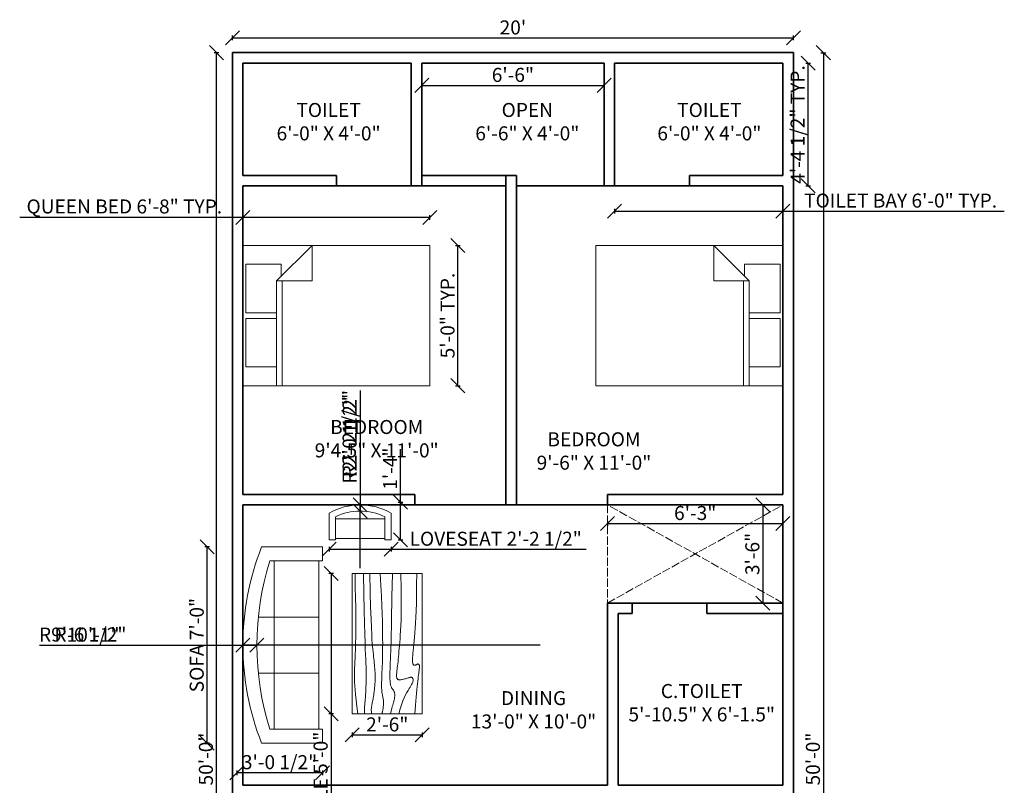
# Model space of a CAD drawing. Units: inches. Extents: x 2598 to 3019, y 330 to 985.
# Tile 2 of 2: x 2598 to 3019, y 657 to 985. Entities that reach past the tile are written whole.
import ezdxf

# ---------------------------------------------------------------- set-up
doc = ezdxf.new("R2010")
doc.units = ezdxf.units.IN
doc.linetypes.add('ACAD_ISO02W100', pattern=[15, 12, -3])
for name, color, linetype, lineweight in [('A-ANNO-DIMS', 2, 'Continuous', 13), ('A-AREA-IDEN', 114, 'Continuous', 18), ('A-FLOR-OVHD', 8, 'ACAD_ISO02W100', 13), ('A-FURN', 8, 'Continuous', 18), ('A-WALL', 7, 'Continuous', 35)]:
    doc.layers.add(name, color=color, linetype=linetype, lineweight=lineweight)
doc.styles.get("Standard").update_dxf_attribs({"font": 'arial.ttf'})
doc.dimstyles.new('ISO-25', dxfattribs={"dimtxt": 6, "dimasz": 6, "dimexe": 1, "dimexo": 3, "dimtad": 1, "dimlunit": 3, "dimtxsty": 'Standard', "dimblk": 'OBLIQUE', "dimcen": 2.5, "dimclrt": 6, "dimadec": 0, "dimazin": 0, "dimtfac": 1, "dimtmove": 0, "dimatfit": 3, "dimfxl": 1, "dimfxlon": 1, "dimarcsym": 0})

# ---------------------------------------------------------------- blocks, each defined once
blk = doc.blocks.new('_Oblique')
at = {"color": 0, "linetype": 'ByBlock', "lineweight": -2}
blk.add_line((-0.5, -0.5), (0.5, 0.5), dxfattribs=at)
blk = doc.blocks.new('*D2')
at = {"layer": 'A-ANNO-DIMS', "color": 0, "lineweight": -2, "transparency": 16777216}
for p, q in [((2770.06, 957.96), (2770.06, 955.96)), ((2770.06, 956.96), (2848.06, 956.96)), ((2848.06, 957.96), (2848.06, 955.96))]:
    blk.add_line(p, q, dxfattribs=at)
at = {"layer": 'Defpoints', "color": 0, "transparency": 16777216}
for p in [(2770.06, 966.44), (2848.06, 966.44), (2848.06, 956.96)]:
    blk.add_point(p, dxfattribs=at)
at = {"layer": 'A-ANNO-DIMS', "color": 0, "lineweight": -2, "transparency": 16777216, "xscale": 6, "yscale": 6, "zscale": 6, "rotation": 180}
blk.add_blockref('_Oblique', (2770.06, 956.96), dxfattribs=at)
at = {"layer": 'A-ANNO-DIMS', "color": 0, "lineweight": -2, "transparency": 16777216, "xscale": 6, "yscale": 6, "zscale": 6}
blk.add_blockref('_Oblique', (2848.06, 956.96), dxfattribs=at)
at = {"layer": 'A-ANNO-DIMS', "color": 0, "transparency": 16777216, "insert": (2809.06, 960.65), "char_height": 6, "attachment_point": 5}
blk.add_mtext('6\'-6"', dxfattribs=at)
blk = doc.blocks.new('*D3')
at = {"layer": 'A-ANNO-DIMS', "color": 0, "lineweight": -2, "transparency": 16777216}
for p, q in [((2689.06, 976.27), (2689.06, 978.27)), ((2929.06, 976.27), (2929.06, 978.27)), ((2689.06, 977.27), (2929.06, 977.27))]:
    blk.add_line(p, q, dxfattribs=at)
at = {"layer": 'Defpoints', "color": 0, "transparency": 16777216}
for p in [(2929.06, 977.27), (2689.06, 970.94), (2929.06, 970.94)]:
    blk.add_point(p, dxfattribs=at)
at = {"layer": 'A-ANNO-DIMS', "color": 0, "lineweight": -2, "transparency": 16777216, "xscale": 6, "yscale": 6, "zscale": 6, "rotation": 180}
blk.add_blockref('_Oblique', (2689.06, 977.27), dxfattribs=at)
at = {"layer": 'A-ANNO-DIMS', "color": 0, "lineweight": -2, "transparency": 16777216, "xscale": 6, "yscale": 6, "zscale": 6}
blk.add_blockref('_Oblique', (2929.06, 977.27), dxfattribs=at)
at = {"layer": 'A-ANNO-DIMS', "color": 0, "transparency": 16777216, "insert": (2809.06, 980.96), "char_height": 6, "attachment_point": 5}
blk.add_mtext("20'", dxfattribs=at)
blk = doc.blocks.new('*D4')
at = {"layer": 'A-ANNO-DIMS', "color": 0, "lineweight": -2, "transparency": 16777216}
for p, q in [((2940.88, 970.94), (2942.88, 970.94)), ((2941.88, 970.94), (2941.88, 366.44)), ((2940.88, 366.44), (2942.88, 366.44))]:
    blk.add_line(p, q, dxfattribs=at)
at = {"layer": 'Defpoints', "color": 0, "transparency": 16777216}
for p in [(2929.06, 970.94), (2929.06, 366.44), (2941.88, 366.44)]:
    blk.add_point(p, dxfattribs=at)
at = {"layer": 'A-ANNO-DIMS', "color": 0, "lineweight": -2, "transparency": 16777216, "xscale": 6, "yscale": 6, "zscale": 6}
for p, rotation in [((2941.88, 970.94), 90), ((2941.88, 366.44), 270)]:
    blk.add_blockref('_Oblique', p, dxfattribs=dict(at, rotation=rotation))
at = {"layer": 'A-ANNO-DIMS', "color": 0, "transparency": 16777216, "insert": (2938.2, 668.69), "char_height": 6, "attachment_point": 5, "rotation": 90}
blk.add_mtext('50\'-0"', dxfattribs=at)
blk = doc.blocks.new('*D7')
at = {"layer": 'A-ANNO-DIMS', "color": 0, "lineweight": -2, "transparency": 16777216}
for p, q in [((2849.56, 770.49), (2849.56, 768.49)), ((2849.56, 769.49), (2924.56, 769.49)), ((2924.56, 770.49), (2924.56, 768.49))]:
    blk.add_line(p, q, dxfattribs=at)
at = {"layer": 'Defpoints', "color": 0, "transparency": 16777216}
for p in [(2849.56, 777.44), (2924.56, 777.44), (2924.56, 769.49)]:
    blk.add_point(p, dxfattribs=at)
at = {"layer": 'A-ANNO-DIMS', "color": 0, "lineweight": -2, "transparency": 16777216, "xscale": 6, "yscale": 6, "zscale": 6, "rotation": 180}
blk.add_blockref('_Oblique', (2849.56, 769.49), dxfattribs=at)
at = {"layer": 'A-ANNO-DIMS', "color": 0, "lineweight": -2, "transparency": 16777216, "xscale": 6, "yscale": 6, "zscale": 6}
blk.add_blockref('_Oblique', (2924.56, 769.49), dxfattribs=at)
at = {"layer": 'A-ANNO-DIMS', "color": 0, "transparency": 16777216, "insert": (2887.06, 773.18), "char_height": 6, "attachment_point": 5}
blk.add_mtext('6\'-3"', dxfattribs=at)
blk = doc.blocks.new('*D8')
at = {"layer": 'A-ANNO-DIMS', "color": 0, "lineweight": -2, "transparency": 16777216}
for p, q in [((2916.98, 777.44), (2914.98, 777.44)), ((2915.98, 777.44), (2915.98, 735.44)), ((2916.98, 735.44), (2914.98, 735.44))]:
    blk.add_line(p, q, dxfattribs=at)
at = {"layer": 'Defpoints', "color": 0, "transparency": 16777216}
for p in [(2924.56, 777.44), (2915.98, 735.44), (2924.56, 735.44)]:
    blk.add_point(p, dxfattribs=at)
at = {"layer": 'A-ANNO-DIMS', "color": 0, "lineweight": -2, "transparency": 16777216, "xscale": 6, "yscale": 6, "zscale": 6}
for p, rotation in [((2915.98, 777.44), 90), ((2915.98, 735.44), 270)]:
    blk.add_blockref('_Oblique', p, dxfattribs=dict(at, rotation=rotation))
at = {"layer": 'A-ANNO-DIMS', "color": 0, "transparency": 16777216, "insert": (2912.29, 756.44), "char_height": 6, "attachment_point": 5, "rotation": 90}
blk.add_mtext('3\'-6"', dxfattribs=at)
blk = doc.blocks.new('Bed - Queen')
for p, q in [((0, -80.00003), (0, 0)), ((0, 0), (59.99999, 0)), ((59.99999, 0), (59.99999, -80.00003)), ((7.99999, -1.2), (28.79998, -1.2)), ((7.99999, -14.4), (7.99999, -1.2)), ((28.79998, -1.2), (28.79998, -14.4)), ((31.19999, -1.2), (51.99999, -1.2)), ((31.19999, -14.4), (31.19999, -1.2)), ((51.99999, -1.2), (51.99999, -16.4)), ((0, -14.4), (44.8, -14.4)), ((44.8, -16.8), (0, -16.8)), ((59.99999, -29.6), (44.8, -14.4)), ((44.8, -14.4), (44.8, -29.6)), ((51.99999, -16.4), (46.79936, -16.4)), ((44.8, -29.6), (59.99999, -29.6)), ((59.99999, -80.00003), (0, -80.00003))]:
    blk.add_line(p, q)
blk = doc.blocks.new('Sofa - Roundback 7 ft.')
for p, q in [((-12.00002, -32.4421), (-12.00003, -6.5971)), ((11.99997, -32.4421), (11.99998, -6.5971)), ((-36.000027, -34), (-36.000027, -11.4696)), ((35.99998, -34), (35.99998, -11.4696)), ((-35.999844, -13.3819), (35.9998, -13.3819)), ((-36.000027, -32.4421), (35.99998, -32.4421))]:
    blk.add_line(p, q)
for points in [[(-36.000027, -34), (-42.000027, -34), (-42.000027, -8)], [(41.99998, -8), (41.99998, -34), (35.99998, -34)]]:
    blk.add_lwpolyline(points)
for centre, radius, start, end in [((0, -114.25), 114.25, 68.43141, 111.5686), ((-0.00001, -127.1968), 121.1968, 72.72033, 107.2797)]:
    blk.add_arc(centre, radius, start, end)
blk = doc.blocks.new('Sofa - Roundback Loveseat 5 ft.')
for p, q in [((0, -32.44198), (0, -5.99998)), ((-24, -33.99998), (-24, -11.46958)), ((-23.9998, -13.38178), (23.99986, -13.38178)), ((24.00004, -33.99998), (24.00004, -11.46958)), ((-24, -32.44198), (24.00004, -32.44198))]:
    blk.add_line(p, q)
for points in [[(-24, -33.99998), (-30, -33.99998), (-30, -7.99998)], [(30.00004, -7.99998), (30.00004, -33.99998), (24.00004, -33.99998)]]:
    blk.add_lwpolyline(points)
for centre, radius, start, end in [((0, -60.24998), 60.24998, 60.13715, 119.8628), ((0, -61.38438), 55.38444, 64.32083, 115.6792)]:
    blk.add_arc(centre, radius, start, end)
blk = doc.blocks.new('Table - Rectangular Woodgrain 60 x 30 in.')
for p, q in [((0, 0), (0, -30)), ((60, 0), (0, 0)), ((60, -30), (60, 0)), ((0, -30), (60, -30))]:
    blk.add_line(p, q)
for points in [[(0, -2.4), (4.8155, -2.418), (9.0302, -2.4688), (12.709, -2.5477), (15.9167, -2.65), (18.7181, -2.7711), (21.1781, -2.9063), (23.3616, -3.0508), (25.3333, -3.2), (27.1477, -3.3495), (28.8172, -3.4958), (30.3437, -3.636), (31.7291, -3.7667), (32.9756, -3.8849), (34.0849, -3.9875), (35.059, -4.0714), (35.9, -4.1334), (36.6114, -4.1711), (37.2041, -4.1854), (37.6906, -4.1779), (38.0833, -4.15), (38.3948, -4.1034), (38.6375, -4.0396), (38.8239, -3.9602), (38.9666, -3.8667), (39.0764, -3.7608), (39.1573, -3.6448), (39.2116, -3.521), (39.2416, -3.3917), (39.2498, -3.2593), (39.2385, -3.1261), (39.21, -2.9944), (39.1666, -2.8667), (39.111, -2.7447), (39.0468, -2.6281), (38.978, -2.5163), (38.9083, -2.4083), (38.8418, -2.3035), (38.7823, -2.201), (38.7337, -2.1001), (38.7, -2), (38.6844, -1.9003), (38.6875, -1.8021), (38.7094, -1.707), (38.75, -1.6167), (38.8094, -1.5326), (38.8875, -1.4563), (38.9844, -1.3893), (39.1, -1.3333), (39.2351, -1.2896), (39.3937, -1.2583), (39.5804, -1.2396), (39.8, -1.2333), (40.057, -1.2396), (40.3562, -1.2583), (40.7023, -1.2896), (41.1, -1.3333), (41.5547, -1.3895), (42.0755, -1.4573), (42.6721, -1.5361), (43.3542, -1.625), (44.1316, -1.7233), (45.014, -1.8302), (46.0114, -1.9449), (47.1333, -2.0667), (48.3862, -2.1947), (49.7625, -2.3281), (51.2513, -2.4663), (52.8416, -2.6083), (54.5226, -2.7535), (56.2833, -2.9011), (58.1127, -3.0501), (60, -3.2)], [(0, -9.2), (6.5759, -9.0858), (11.9385, -9.0365), (16.2527, -9.0418), (19.6833, -9.0917), (22.3952, -9.1759), (24.5531, -9.2844), (26.322, -9.4069), (27.8666, -9.5333), (29.3241, -9.6553), (30.7203, -9.7719), (32.0532, -9.8837), (33.3208, -9.9917), (34.5213, -10.0965), (35.6526, -10.199), (36.7128, -10.2999), (37.7, -10.4), (38.6129, -10.4996), (39.4531, -10.5969), (40.223, -10.6895), (40.925, -10.775), (41.5613, -10.8512), (42.1344, -10.9156), (42.6465, -10.966), (43.1, -11), (43.4976, -11.0158), (43.8437, -11.0136), (44.143, -10.9942), (44.4, -10.9583), (44.6195, -10.9069), (44.8062, -10.8406), (44.9648, -10.7603), (45.1, -10.6667), (45.2155, -10.5598), (45.3114, -10.4365), (45.3871, -10.2929), (45.4416, -10.125), (45.4743, -9.929), (45.4844, -9.7011), (45.4709, -9.4371), (45.4333, -9.1333), (45.3716, -8.7883), (45.2896, -8.4104), (45.1919, -8.0107), (45.0833, -7.6), (44.9685, -7.1893), (44.8521, -6.7896), (44.7388, -6.4117), (44.6333, -6.0667), (44.54, -5.7628), (44.4614, -5.4979), (44.4001, -5.2675), (44.3583, -5.0667), (44.3384, -4.8909), (44.3427, -4.7354), (44.3736, -4.5956), (44.4333, -4.4667), (44.5236, -4.3453), (44.6427, -4.2333), (44.7884, -4.1339), (44.9583, -4.05), (45.1501, -3.9849), (45.3614, -3.9417), (45.59, -3.9234), (45.8333, -3.9333), (46.0915, -3.9749), (46.3734, -4.0531), (46.6906, -4.1736), (47.0542, -4.3417), (47.4756, -4.5629), (47.9661, -4.8427), (48.5372, -5.1866), (49.2, -5.6), (49.9676, -6.0844), (50.8594, -6.625), (51.8965, -7.2031), (53.1, -7.8), (54.491, -8.3969), (56.0906, -8.975), (57.9199, -9.5156), (60, -10)], [(0, -12.8), (5.1847, -12.9322), (9.6213, -13.0323), (13.3963, -13.1059), (16.5958, -13.1583), (19.3063, -13.1952), (21.614, -13.2219), (23.6054, -13.2439), (25.3666, -13.2667), (26.9728, -13.2947), (28.4531, -13.3281), (29.8256, -13.3663), (31.1083, -13.4083), (32.3191, -13.4535), (33.476, -13.501), (34.597, -13.5501), (35.7, -13.6), (36.7984, -13.6497), (37.8875, -13.6979), (38.9578, -13.743), (40, -13.7833), (41.0047, -13.8174), (41.9625, -13.8438), (42.864, -13.8607), (43.7, -13.8667), (44.4631, -13.8604), (45.1552, -13.8417), (45.7801, -13.8104), (46.3416, -13.7667), (46.8439, -13.7104), (47.2906, -13.6417), (47.6858, -13.5604), (48.0333, -13.4667), (48.3375, -13.3608), (48.6042, -13.2448), (48.8396, -13.121), (49.05, -12.9917), (49.2417, -12.8593), (49.4208, -12.7261), (49.5937, -12.5944), (49.7667, -12.4667), (49.9452, -12.3451), (50.1323, -12.2313), (50.3303, -12.1268), (50.5416, -12.0333), (50.7686, -11.9524), (51.0135, -11.8854), (51.2788, -11.8341), (51.5666, -11.8), (51.8785, -11.7843), (52.2116, -11.7865), (52.562, -11.8059), (52.926, -11.8417), (53.2998, -11.8931), (53.6795, -11.9594), (54.0614, -12.0397), (54.4416, -12.1333), (54.8223, -12.2401), (55.2293, -12.3625), (55.6942, -12.5037), (56.2489, -12.6667), (56.9251, -12.8547), (57.7545, -13.0708), (58.7689, -13.3182), (60, -13.6)], [(0, -18), (5.124, -17.7273), (9.6609, -17.5057), (13.6705, -17.3303), (17.2125, -17.1958), (20.3467, -17.0973), (23.1328, -17.0297), (25.6307, -16.9878), (27.9, -16.9667), (29.9928, -16.9617), (31.9302, -16.9703), (33.7254, -16.9907), (35.3917, -17.0208), (36.9423, -17.0588), (38.3906, -17.1026), (39.7499, -17.1503), (41.0333, -17.2), (42.2519, -17.2496), (43.4073, -17.2969), (44.4986, -17.3395), (45.525, -17.375), (46.4858, -17.4012), (47.3802, -17.4156), (48.2074, -17.416), (48.9667, -17.4), (49.6583, -17.3662), (50.2872, -17.3167), (50.8595, -17.2547), (51.3812, -17.1833), (51.8584, -17.1057), (52.2971, -17.025), (52.7034, -16.9443), (53.0833, -16.8667), (53.443, -16.7951), (53.789, -16.7313), (54.128, -16.6768), (54.4666, -16.6334), (54.8115, -16.6024), (55.1693, -16.5854), (55.5465, -16.5841), (55.95, -16.6), (56.3828, -16.6337), (56.8346, -16.6823), (57.2915, -16.7418), (57.7396, -16.8084), (58.165, -16.878), (58.5539, -16.9469), (58.8924, -17.0111), (59.1666, -17.0667), (59.3679, -17.1107), (59.5078, -17.1438), (59.6032, -17.1675), (59.6708, -17.1833), (59.7275, -17.193), (59.7901, -17.1979), (59.8753, -17.1998), (60, -17.2)], [(0, -22.4), (8.0098, -22.2501), (14.4094, -22.1011), (19.4168, -21.9535), (23.25, -21.8083), (26.1269, -21.6663), (28.2656, -21.5281), (29.884, -21.3947), (31.2, -21.2667), (32.3967, -21.1448), (33.5172, -21.0292), (34.5697, -20.9198), (35.5625, -20.8167), (36.5037, -20.7198), (37.4015, -20.6292), (38.2642, -20.5448), (39.1, -20.4667), (39.9164, -20.3951), (40.7187, -20.3313), (41.5117, -20.2768), (42.3, -20.2333), (43.0883, -20.2024), (43.8812, -20.1854), (44.6836, -20.1841), (45.5, -20.2), (46.3328, -20.234), (47.1747, -20.2844), (48.0163, -20.3488), (48.8479, -20.425), (49.66, -20.5106), (50.4429, -20.6031), (51.1872, -20.7004), (51.8833, -20.8), (52.5246, -20.8999), (53.1166, -20.9995), (53.6681, -21.0983), (54.1875, -21.1958), (54.6834, -21.2919), (55.1646, -21.3859), (55.6394, -21.4777), (56.1167, -21.5667), (56.6028, -21.6515), (57.0961, -21.7266), (57.5929, -21.7852), (58.0896, -21.8208), (58.5823, -21.8268), (59.0674, -21.7964), (59.5412, -21.723), (60, -21.6)], [(0, -25.2), (8.6355, -25.0504), (15.7026, -24.9031), (21.4049, -24.7606), (25.9458, -24.625), (29.529, -24.4988), (32.3578, -24.3844), (34.6359, -24.284), (36.5667, -24.2), (38.3213, -24.1341), (39.9417, -24.0854), (41.437, -24.0523), (42.8167, -24.0333), (44.0901, -24.0268), (45.2667, -24.0313), (46.3557, -24.0451), (47.3667, -24.0667), (48.309, -24.0947), (49.1928, -24.1287), (50.0284, -24.168), (50.826, -24.2125), (51.5959, -24.2617), (52.3483, -24.3151), (53.0935, -24.3725), (53.8417, -24.4334), (54.6009, -24.497), (55.3699, -24.561), (56.1454, -24.6226), (56.9239, -24.6792), (57.7021, -24.7279), (58.4764, -24.7662), (59.2435, -24.7911), (60, -24.8)], [(0, -28.8), (5.6867, -28.6681), (10.45, -28.5698), (14.407, -28.5012), (17.675, -28.4584), (20.3711, -28.4374), (22.6125, -28.4344), (24.5164, -28.4455), (26.2, -28.4667), (27.762, -28.4947), (29.2276, -28.5281), (30.6033, -28.5663), (31.8958, -28.6084), (33.1118, -28.6535), (34.2578, -28.7011), (35.3405, -28.7501), (36.3666, -28.8), (37.3443, -28.8497), (38.288, -28.8974), (39.2137, -28.9412), (40.1375, -28.9792), (41.0753, -29.0093), (42.0432, -29.0297), (43.0572, -29.0384), (44.1333, -29.0333), (45.2936, -29.0114), (46.5843, -28.9641), (48.0579, -28.8816), (49.7666, -28.7542), (51.7629, -28.5721), (54.0989, -28.3255), (56.8272, -28.0048), (60, -27.6)]]:
    blk.add_lwpolyline(points)
blk = doc.blocks.new('*D15')
at = {"layer": 'A-ANNO-DIMS', "color": 0, "lineweight": -2, "transparency": 16777216}
for p, q in [((2683.19, 970.94), (2681.19, 970.94)), ((2682.19, 366.44), (2682.19, 970.94)), ((2683.19, 366.44), (2681.19, 366.44))]:
    blk.add_line(p, q, dxfattribs=at)
at = {"layer": 'Defpoints', "color": 0, "transparency": 16777216}
for p in [(2682.19, 970.94), (2689.06, 970.94), (2689.06, 366.44)]:
    blk.add_point(p, dxfattribs=at)
at = {"layer": 'A-ANNO-DIMS', "color": 0, "lineweight": -2, "transparency": 16777216, "xscale": 6, "yscale": 6, "zscale": 6}
for p, rotation in [((2682.19, 970.94), 90), ((2682.19, 366.44), 270)]:
    blk.add_blockref('_Oblique', p, dxfattribs=dict(at, rotation=rotation))
at = {"layer": 'A-ANNO-DIMS', "color": 0, "transparency": 16777216, "insert": (2678.5, 668.69), "char_height": 6, "attachment_point": 5, "rotation": 90}
blk.add_mtext('50\'-0"', dxfattribs=at)
blk = doc.blocks.new('TOILET-BAY-WALL-72X48')
for p, q in [((72, 52.5), (0, 52.5)), ((0, 52.5), (0, 0)), ((72, 4.5), (72, 52.5)), ((72, 4.5), (32, 4.5)), ((32, 4.5), (32, 0))]:
    blk.add_line(p, q)
blk = doc.blocks.new('*D17')
at = {"layer": 'A-ANNO-DIMS', "color": 0, "lineweight": -2, "transparency": 16777216}
for p, q in [((2693.56, 900.45), (2598.05, 900.45)), ((2693.56, 899.45), (2693.56, 901.45)), ((2773.56, 900.45), (2693.56, 900.45)), ((2773.56, 899.45), (2773.56, 901.45))]:
    blk.add_line(p, q, dxfattribs=at)
at = {"layer": 'Defpoints', "color": 0, "transparency": 16777216}
for p in [(2693.56, 900.45), (2693.56, 888.45), (2773.56, 888.45)]:
    blk.add_point(p, dxfattribs=at)
at = {"layer": 'A-ANNO-DIMS', "color": 0, "lineweight": -2, "transparency": 16777216, "xscale": 6, "yscale": 6, "zscale": 6, "rotation": 180}
blk.add_blockref('_Oblique', (2693.56, 900.45), dxfattribs=at)
at = {"layer": 'A-ANNO-DIMS', "color": 0, "lineweight": -2, "transparency": 16777216, "xscale": 6, "yscale": 6, "zscale": 6}
blk.add_blockref('_Oblique', (2773.56, 900.45), dxfattribs=at)
at = {"layer": 'A-ANNO-DIMS', "color": 6, "transparency": 16777216, "insert": (2642.81, 904.36), "char_height": 6, "attachment_point": 5}
blk.add_mtext('QUEEN BED 6\'-8" TYP.', dxfattribs=at)
blk = doc.blocks.new('*D18')
at = {"layer": 'A-ANNO-DIMS', "color": 0, "lineweight": -2, "transparency": 16777216}
for p, q in [((2784.56, 888.45), (2786.56, 888.45)), ((2785.56, 828.45), (2785.56, 888.45)), ((2784.56, 828.45), (2786.56, 828.45))]:
    blk.add_line(p, q, dxfattribs=at)
at = {"layer": 'Defpoints', "color": 0, "transparency": 16777216}
for p in [(2773.56, 888.45), (2785.56, 888.45), (2773.56, 828.45)]:
    blk.add_point(p, dxfattribs=at)
at = {"layer": 'A-ANNO-DIMS', "color": 0, "lineweight": -2, "transparency": 16777216, "xscale": 6, "yscale": 6, "zscale": 6}
for p, rotation in [((2785.56, 888.45), 90), ((2785.56, 828.45), 270)]:
    blk.add_blockref('_Oblique', p, dxfattribs=dict(at, rotation=rotation))
at = {"layer": 'A-ANNO-DIMS', "color": 6, "transparency": 16777216, "insert": (2781.87, 858.45), "char_height": 6, "attachment_point": 5, "rotation": 90}
blk.add_mtext('5\'-0" TYP.', dxfattribs=at)
blk = doc.blocks.new('*D19')
at = {"layer": 'A-ANNO-DIMS', "color": 0, "lineweight": -2, "transparency": 16777216}
for p, q in [((2852.56, 904.14), (2852.56, 902.14)), ((2852.56, 903.14), (2924.56, 903.14)), ((2924.56, 904.14), (2924.56, 902.14)), ((2924.56, 903.14), (3019.31, 903.14))]:
    blk.add_line(p, q, dxfattribs=at)
at = {"layer": 'Defpoints', "color": 0, "transparency": 16777216}
for p in [(2852.56, 913.94), (2924.56, 913.94), (2924.56, 903.14)]:
    blk.add_point(p, dxfattribs=at)
at = {"layer": 'A-ANNO-DIMS', "color": 0, "lineweight": -2, "transparency": 16777216, "xscale": 6, "yscale": 6, "zscale": 6, "rotation": 180}
blk.add_blockref('_Oblique', (2852.56, 903.14), dxfattribs=at)
at = {"layer": 'A-ANNO-DIMS', "color": 0, "lineweight": -2, "transparency": 16777216, "xscale": 6, "yscale": 6, "zscale": 6}
blk.add_blockref('_Oblique', (2924.56, 903.14), dxfattribs=at)
at = {"layer": 'A-ANNO-DIMS', "color": 6, "transparency": 16777216, "insert": (2974.93, 906.87), "char_height": 6, "attachment_point": 5}
blk.add_mtext('TOILET BAY 6\'-0" TYP.', dxfattribs=at)
blk = doc.blocks.new('*D20')
at = {"layer": 'A-ANNO-DIMS', "color": 0, "lineweight": -2, "transparency": 16777216}
for p, q in [((2934.36, 966.44), (2936.36, 966.44)), ((2935.36, 913.94), (2935.36, 966.44)), ((2934.36, 913.94), (2936.36, 913.94))]:
    blk.add_line(p, q, dxfattribs=at)
at = {"layer": 'Defpoints', "color": 0, "transparency": 16777216}
for p in [(2924.56, 966.44), (2935.36, 966.44), (2924.56, 913.94)]:
    blk.add_point(p, dxfattribs=at)
at = {"layer": 'A-ANNO-DIMS', "color": 0, "lineweight": -2, "transparency": 16777216, "xscale": 6, "yscale": 6, "zscale": 6}
for p, rotation in [((2935.36, 966.44), 90), ((2935.36, 913.94), 270)]:
    blk.add_blockref('_Oblique', p, dxfattribs=dict(at, rotation=rotation))
at = {"layer": 'A-ANNO-DIMS', "color": 6, "transparency": 16777216, "insert": (2931.63, 940.19), "char_height": 6, "attachment_point": 5, "rotation": 90}
blk.add_mtext('4\'-4 1/2" TYP.', dxfattribs=at)
blk = doc.blocks.new('*D21')
at = {"layer": 'A-ANNO-DIMS', "color": 0, "lineweight": -2, "transparency": 16777216}
for p, q in [((2679.29, 759.44), (2677.29, 759.44)), ((2678.29, 675.44), (2678.29, 759.44)), ((2679.29, 675.44), (2677.29, 675.44))]:
    blk.add_line(p, q, dxfattribs=at)
at = {"layer": 'Defpoints', "color": 0, "transparency": 16777216}
for p in [(2678.29, 759.44), (2690.89, 759.44), (2690.89, 675.44)]:
    blk.add_point(p, dxfattribs=at)
at = {"layer": 'A-ANNO-DIMS', "color": 0, "lineweight": -2, "transparency": 16777216, "xscale": 6, "yscale": 6, "zscale": 6}
for p, rotation in [((2678.29, 759.44), 90), ((2678.29, 675.44), 270)]:
    blk.add_blockref('_Oblique', p, dxfattribs=dict(at, rotation=rotation))
at = {"layer": 'A-ANNO-DIMS', "color": 6, "transparency": 16777216, "insert": (2674.57, 717.44), "char_height": 6, "attachment_point": 5, "rotation": 90}
blk.add_mtext('SOFA 7\'-0"', dxfattribs=at)
blk = doc.blocks.new('*D22')
at = {"layer": 'A-ANNO-DIMS', "color": 0, "lineweight": -2, "transparency": 16777216}
for p, q in [((2690.89, 663.84), (2690.89, 661.84)), ((2727.56, 662.84), (2690.89, 662.84)), ((2727.56, 663.84), (2727.56, 661.84))]:
    blk.add_line(p, q, dxfattribs=at)
at = {"layer": 'Defpoints', "color": 0, "transparency": 16777216}
for p in [(2690.89, 675.44), (2727.56, 675.44), (2690.89, 662.84)]:
    blk.add_point(p, dxfattribs=at)
at = {"layer": 'A-ANNO-DIMS', "color": 0, "lineweight": -2, "transparency": 16777216, "xscale": 6, "yscale": 6, "zscale": 6, "rotation": 180}
blk.add_blockref('_Oblique', (2690.89, 662.84), dxfattribs=at)
at = {"layer": 'A-ANNO-DIMS', "color": 0, "lineweight": -2, "transparency": 16777216, "xscale": 6, "yscale": 6, "zscale": 6}
blk.add_blockref('_Oblique', (2727.56, 662.84), dxfattribs=at)
at = {"layer": 'A-ANNO-DIMS', "color": 6, "transparency": 16777216, "insert": (2709.23, 666.57), "char_height": 6, "attachment_point": 5}
blk.add_mtext('3\'-0 1/2"', dxfattribs=at)
blk = doc.blocks.new('*D23')
at = {"layer": 'A-ANNO-DIMS', "color": 0, "lineweight": -2, "transparency": 16777216}
for p, q in [((2730.46, 759.42), (2730.46, 757.45)), ((2730.46, 758.45), (2756.96, 758.45)), ((2756.96, 759.42), (2756.96, 757.45)), ((2756.96, 758.45), (2840.46, 758.45))]:
    blk.add_line(p, q, dxfattribs=at)
at = {"layer": 'Defpoints', "color": 0, "transparency": 16777216}
for p in [(2730.46, 762.42), (2756.96, 762.42), (2756.96, 758.45)]:
    blk.add_point(p, dxfattribs=at)
at = {"layer": 'A-ANNO-DIMS', "color": 0, "lineweight": -2, "transparency": 16777216, "xscale": 6, "yscale": 6, "zscale": 6, "rotation": 180}
blk.add_blockref('_Oblique', (2730.46, 758.45), dxfattribs=at)
at = {"layer": 'A-ANNO-DIMS', "color": 0, "lineweight": -2, "transparency": 16777216, "xscale": 6, "yscale": 6, "zscale": 6}
blk.add_blockref('_Oblique', (2756.96, 758.45), dxfattribs=at)
at = {"layer": 'A-ANNO-DIMS', "color": 6, "transparency": 16777216, "insert": (2801.71, 762.18), "char_height": 6, "attachment_point": 5}
blk.add_mtext('LOVESEAT 2\'-2 1/2"', dxfattribs=at)
blk = doc.blocks.new('*D24')
at = {"layer": 'A-ANNO-DIMS', "color": 0, "lineweight": -2, "transparency": 16777216}
for p, q in [((2760.94, 778.62), (2760.94, 801.26)), ((2759.96, 778.62), (2761.94, 778.62)), ((2760.94, 762.42), (2760.94, 778.62)), ((2759.96, 762.42), (2761.94, 762.42))]:
    blk.add_line(p, q, dxfattribs=at)
at = {"layer": 'Defpoints', "color": 0, "transparency": 16777216}
for p in [(2756.96, 778.62), (2760.94, 778.62), (2756.96, 762.42)]:
    blk.add_point(p, dxfattribs=at)
at = {"layer": 'A-ANNO-DIMS', "color": 0, "lineweight": -2, "transparency": 16777216, "xscale": 6, "yscale": 6, "zscale": 6}
for p, rotation in [((2760.94, 778.62), 90), ((2760.94, 762.42), 270)]:
    blk.add_blockref('_Oblique', p, dxfattribs=dict(at, rotation=rotation))
at = {"layer": 'A-ANNO-DIMS', "color": 6, "transparency": 16777216, "insert": (2757.3, 792.94), "char_height": 6, "attachment_point": 5, "rotation": 90}
blk.add_mtext('1\'-4"', dxfattribs=at)
blk = doc.blocks.new('*D25')
at = {"layer": 'A-ANNO-DIMS', "color": 0, "lineweight": -2, "transparency": 16777216}
for p, q in [((2732.31, 748.04), (2730.31, 748.04)), ((2731.31, 748.04), (2731.31, 688.04)), ((2732.31, 688.04), (2730.31, 688.04)), ((2731.31, 688.04), (2731.31, 604.59))]:
    blk.add_line(p, q, dxfattribs=at)
at = {"layer": 'Defpoints', "color": 0, "transparency": 16777216}
for p in [(2740.31, 748.04), (2731.31, 688.04), (2740.31, 688.04)]:
    blk.add_point(p, dxfattribs=at)
at = {"layer": 'A-ANNO-DIMS', "color": 0, "lineweight": -2, "transparency": 16777216, "xscale": 6, "yscale": 6, "zscale": 6}
for p, rotation in [((2731.31, 748.04), 90), ((2731.31, 688.04), 270)]:
    blk.add_blockref('_Oblique', p, dxfattribs=dict(at, rotation=rotation))
at = {"layer": 'A-ANNO-DIMS', "color": 6, "transparency": 16777216, "insert": (2727.58, 643.32), "char_height": 6, "attachment_point": 5, "rotation": 90}
blk.add_mtext('DINING TABLE 5\'-0"', dxfattribs=at)
blk = doc.blocks.new('*D26')
at = {"layer": 'A-ANNO-DIMS', "color": 0, "lineweight": -2, "transparency": 16777216}
for p, q in [((2740.31, 680.04), (2740.31, 678.04)), ((2740.31, 679.04), (2770.31, 679.04)), ((2770.31, 680.04), (2770.31, 678.04))]:
    blk.add_line(p, q, dxfattribs=at)
at = {"layer": 'Defpoints', "color": 0, "transparency": 16777216}
for p in [(2740.31, 688.04), (2770.31, 688.04), (2770.31, 679.04)]:
    blk.add_point(p, dxfattribs=at)
at = {"layer": 'A-ANNO-DIMS', "color": 0, "lineweight": -2, "transparency": 16777216, "xscale": 6, "yscale": 6, "zscale": 6, "rotation": 180}
blk.add_blockref('_Oblique', (2740.31, 679.04), dxfattribs=at)
at = {"layer": 'A-ANNO-DIMS', "color": 0, "lineweight": -2, "transparency": 16777216, "xscale": 6, "yscale": 6, "zscale": 6}
blk.add_blockref('_Oblique', (2770.31, 679.04), dxfattribs=at)
at = {"layer": 'A-ANNO-DIMS', "color": 6, "transparency": 16777216, "insert": (2755.31, 682.73), "char_height": 6, "attachment_point": 5}
blk.add_mtext('2\'-6"', dxfattribs=at)
blk = doc.blocks.new('*D35')
at = {"layer": 'A-ANNO-DIMS', "color": 0, "lineweight": -2, "transparency": 16777216}
for p in [(2613.04, 717.45), (2820.76, 717.44)]:
    blk.add_line(p, (2699.56, 717.44), dxfattribs=at)
at = {"layer": 'Defpoints', "color": 0, "transparency": 16777216}
for p in [(2699.56, 717.44), (2820.76, 717.44)]:
    blk.add_point(p, dxfattribs=at)
at = {"layer": 'A-ANNO-DIMS', "color": 0, "lineweight": -2, "transparency": 16777216, "xscale": 6, "yscale": 6, "zscale": 6, "rotation": 359.9998109000254}
blk.add_blockref('_Oblique', (2699.56, 717.44), dxfattribs=at)
at = {"layer": 'A-ANNO-DIMS', "color": 6, "transparency": 16777216, "insert": (2626.84, 721.13), "char_height": 6, "attachment_point": 5, "rotation": 359.9998}
blk.add_mtext('R10\'-1"', dxfattribs=at)
blk = doc.blocks.new('*D36')
at = {"layer": 'A-ANNO-DIMS', "color": 0, "lineweight": -2, "transparency": 16777216}
for p in [(2606.55, 717.45), (2807.81, 717.44)]:
    blk.add_line(p, (2693.56, 717.45), dxfattribs=at)
at = {"layer": 'Defpoints', "color": 0, "transparency": 16777216}
for p in [(2693.56, 717.45), (2807.81, 717.44)]:
    blk.add_point(p, dxfattribs=at)
at = {"layer": 'A-ANNO-DIMS', "color": 0, "lineweight": -2, "transparency": 16777216, "xscale": 6, "yscale": 6, "zscale": 6, "rotation": 359.9998044170326}
blk.add_blockref('_Oblique', (2693.56, 717.45), dxfattribs=at)
at = {"layer": 'A-ANNO-DIMS', "color": 6, "transparency": 16777216, "insert": (2625.01, 721.17), "char_height": 6, "attachment_point": 5, "rotation": 359.9998}
blk.add_mtext('R9\'-6 1/2"', dxfattribs=at)
blk = doc.blocks.new('*D37')
at = {"layer": 'A-ANNO-DIMS', "color": 0, "lineweight": -2, "transparency": 16777216}
for p in [(2743.71, 826.37), (2743.71, 750.83)]:
    blk.add_line(p, (2743.71, 777.44), dxfattribs=at)
at = {"layer": 'Defpoints', "color": 0, "transparency": 16777216}
for p in [(2743.71, 777.44), (2743.71, 750.83)]:
    blk.add_point(p, dxfattribs=at)
at = {"layer": 'A-ANNO-DIMS', "color": 0, "lineweight": -2, "transparency": 16777216, "xscale": 6, "yscale": 6, "zscale": 6, "rotation": 269.9996211338203}
blk.add_blockref('_Oblique', (2743.71, 777.44), dxfattribs=at)
at = {"layer": 'A-ANNO-DIMS', "color": 6, "transparency": 16777216, "insert": (2739.98, 807.91), "char_height": 6, "attachment_point": 5, "rotation": 89.9996}
blk.add_mtext('R2\'-2 1/2"', dxfattribs=at)
blk = doc.blocks.new('*D38')
at = {"layer": 'A-ANNO-DIMS', "color": 0, "lineweight": -2, "transparency": 16777216}
for p in [(2743.71, 823.72), (2743.71, 750.33)]:
    blk.add_line(p, (2743.71, 774.79), dxfattribs=at)
at = {"layer": 'Defpoints', "color": 0, "transparency": 16777216}
for p in [(2743.71, 774.79), (2743.71, 750.33)]:
    blk.add_point(p, dxfattribs=at)
at = {"layer": 'A-ANNO-DIMS', "color": 0, "lineweight": -2, "transparency": 16777216, "xscale": 6, "yscale": 6, "zscale": 6, "rotation": 269.9995878503183}
blk.add_blockref('_Oblique', (2743.71, 774.79), dxfattribs=at)
at = {"layer": 'A-ANNO-DIMS', "color": 6, "transparency": 16777216, "insert": (2739.98, 805.26), "char_height": 6, "attachment_point": 5, "rotation": 89.9996}
blk.add_mtext('R2\'-0 1/2"', dxfattribs=at)

msp = doc.modelspace()

# ---------------------------------------------------------------- linework, layer by layer
at = {"layer": 'A-FLOR-OVHD', "ltscale": 0.3}
for p, q in [((2849.562, 777.445), (2849.562, 735.445)), ((2924.562, 735.445), (2849.562, 777.445)), ((2849.562, 735.445), (2924.562, 777.445))]:
    msp.add_line(p, q, dxfattribs=at)
at = {"layer": 'A-WALL'}
for p, q in [((2929.062, 970.945), (2689.062, 970.945)), ((2689.062, 970.945), (2689.062, 366.445)), ((2929.062, 366.445), (2929.062, 970.945)), ((2770.062, 966.445), (2770.062, 913.945)), ((2848.062, 966.445), (2770.062, 966.445)), ((2848.062, 966.445), (2848.062, 913.945)), ((2810.562, 918.445), (2770.062, 918.445)), ((2806.062, 918.445), (2806.062, 777.445)), ((2810.562, 918.445), (2810.562, 777.445)), ((2693.562, 913.945), (2693.562, 781.945)), ((2806.062, 913.945), (2693.562, 913.945)), ((2924.562, 913.945), (2810.562, 913.945)), ((2924.562, 781.945), (2924.562, 913.945)), ((2767.062, 781.945), (2693.562, 781.945)), ((2767.062, 781.945), (2767.062, 777.445)), ((2924.562, 781.945), (2849.562, 781.945)), ((2849.562, 781.945), (2849.562, 777.445)), ((2693.562, 777.445), (2693.562, 657.445)), ((2849.562, 777.445), (2693.562, 777.445)), ((2924.562, 777.445), (2849.562, 777.445)), ((2924.562, 657.445), (2924.562, 777.445)), ((2924.562, 735.445), (2849.562, 735.445)), ((2849.562, 735.445), (2849.562, 657.445)), ((2860.062, 730.945), (2860.062, 735.445)), ((2892.062, 730.945), (2892.062, 735.445)), ((2854.062, 730.945), (2854.062, 657.445)), ((2860.062, 730.945), (2854.062, 730.945)), ((2924.562, 730.945), (2892.062, 730.945)), ((2849.562, 657.445), (2693.562, 657.445)), ((2924.562, 657.445), (2854.062, 657.445))]:
    msp.add_line(p, q, dxfattribs=at)

# ---------------------------------------------------------------- block references
at = {"layer": 'A-FURN'}
for name, p, rotation in [('Bed - Queen', (2693.562, 828.446), 90), ('Sofa - Roundback 7 ft.', (2693.562, 717.445), 90), ('Table - Rectangular Woodgrain 60 x 30 in.', (2770.309, 748.042), 270)]:
    msp.add_blockref(name, p, dxfattribs=dict(at, rotation=rotation))
at = {"layer": 'A-FURN', "xscale": -1, "rotation": 270}
msp.add_blockref('Bed - Queen', (2924.562, 828.446), dxfattribs=at)
at = {"layer": 'A-FURN', "xscale": 0.4417662769449516, "yscale": 0.4417662769449516, "zscale": 0.4417662769449516}
msp.add_blockref('Sofa - Roundback Loveseat 5 ft.', (2743.71, 777.445), dxfattribs=at)
at = {"layer": 'A-WALL', "extrusion": (0, 0, -1), "zscale": -1}
msp.add_blockref('TOILET-BAY-WALL-72X48', (-2765.561, 913.945), dxfattribs=at)
at = {"layer": 'A-WALL'}
msp.add_blockref('TOILET-BAY-WALL-72X48', (2852.562, 913.945), dxfattribs=at)

# ---------------------------------------------------------------- texts
at = {"layer": 'A-AREA-IDEN', "char_height": 6, "attachment_point": 1}
for s, width, insert in [('\\pxqc;TOILET\\P6\'-0" X 4\'-0"', 66.36505, (2697.023, 949.414)), ('\\pxqc;OPEN\\P6\'-6" X 4\'-0"', 66.36505, (2782.053, 949.414)), ('\\pxqc;TOILET\\P6\'-0" X 4\'-0"', 66.36505, (2859.94, 949.414)), ('\\pxqc;BEDROOM\\P9\'4.5" X 11\'-0"', 66.36505, (2717.611, 813.763)), ('\\pxqc;BEDROOM\\P9\'-6" X 11\'-0"', 66.36505, (2810.562, 808.49)), ('\\pxqc;C.TOILET\\P5\'-10.5" X 6\'-1.5"', 62.70828, (2858.497, 700.787)), ('\\pxqc;DINING\\P13\'-0" X 10\'-0"', 66.36505, (2784.717, 697.76))]:
    msp.add_mtext_dynamic_manual_height_columns(s, width=width, gutter_width=12.5, heights=[0], dxfattribs=dict(at, insert=insert))

# ---------------------------------------------------------------- dimensions: what is measured, and where the dimension line sits
at = {"layer": 'A-ANNO-DIMS'}
for base, p1, p2, override, picture, middle in [((2929.062, 977.274), (2689.062, 970.945), (2929.062, 970.945), {"dimclrd": 0, "dimclre": 0, "dimclrt": 0}, '*D3', (2809.062, 980.963)), ((2848.062, 956.957), (2770.062, 966.445), (2848.062, 966.445), {"dimclrd": 0, "dimclre": 0, "dimclrt": 0}, '*D2', (2809.062, 960.645)), ((2924.562, 769.493), (2849.562, 777.445), (2924.562, 777.445), {"dimclrd": 0, "dimclre": 0, "dimclrt": 0}, '*D7', (2887.062, 773.183)), ((2770.309, 679.042), (2740.309, 688.042), (2770.309, 688.042), {"dimdec": 1, "dimlfac": 1, "dimrnd": 0, "dimzin": 1, "dimdsep": 46, "dimlunit": 4, "dimfrac": 2}, '*D26', (2755.309, 682.73))]:
    dim = msp.add_linear_dim(base=base, p1=p1, p2=p2, dimstyle='ISO-25', override=override, dxfattribs=at)
    dim.commit()
    dim.dimension.update_dxf_attribs({"geometry": picture, "text_midpoint": middle})
for base, p1, p2, angle, text, override, picture, middle in [((2682.187, 970.945), (2689.062, 366.445), (2689.062, 970.945), 90, '50\'-0"', {"dimclrd": 0, "dimclre": 0, "dimclrt": 0}, '*D15', (2678.498, 668.695)), ((2941.884, 366.445), (2929.062, 970.945), (2929.062, 366.445), 90, '50\'-0"', {"dimclrd": 0, "dimclre": 0, "dimclrt": 0}, '*D4', (2938.195, 668.695)), ((2935.362, 966.445), (2924.562, 913.945), (2924.562, 966.445), 90, '<> TYP.', {"dimdec": 1, "dimlfac": 1, "dimrnd": 0, "dimzin": 1, "dimdsep": 46, "dimlunit": 4, "dimfrac": 2}, '*D20', (2931.634, 940.195)), ((2693.562, 900.446), (2773.562, 888.446), (2693.562, 888.446), 180, 'QUEEN BED <> TYP.', {"dimdec": 1, "dimlfac": 1, "dimrnd": 0, "dimzin": 1, "dimdsep": 46, "dimlunit": 4, "dimfrac": 2}, '*D17', (2642.806, 904.357)), ((2785.562, 888.446), (2773.562, 828.446), (2773.562, 888.446), 90, '<> TYP.', {"dimdec": 1, "dimlfac": 1, "dimrnd": 0, "dimzin": 1, "dimdsep": 46, "dimlunit": 4, "dimfrac": 2}, '*D18', (2781.873, 858.446)), ((2678.295, 759.445), (2690.895, 675.445), (2690.895, 759.445), 90, 'SOFA <>', {"dimdec": 1, "dimlfac": 1, "dimrnd": 0, "dimzin": 1, "dimdsep": 46, "dimlunit": 4, "dimfrac": 2}, '*D21', (2674.566, 717.445)), ((2731.309, 688.042), (2740.309, 748.042), (2740.309, 688.042), 270, 'DINING TABLE <>', {"dimdec": 1, "dimlfac": 1, "dimrnd": 0, "dimzin": 1, "dimdsep": 46, "dimlunit": 4, "dimfrac": 2}, '*D25', (2727.582, 643.317))]:
    dim = msp.add_linear_dim(base=base, p1=p1, p2=p2, angle=angle, text=text, dimstyle='ISO-25', override=override, dxfattribs=at)
    dim.commit()
    dim.dimension.update_dxf_attribs({"geometry": picture, "text_midpoint": middle})
for base, p1, p2, text, picture, middle in [((2924.562, 903.145), (2852.562, 913.945), (2924.562, 913.945), 'TOILET BAY <> TYP.', '*D19', (2974.934, 906.874)), ((2756.963, 758.449), (2730.457, 762.425), (2756.963, 762.425), 'LOVESEAT <>', '*D23', (2801.712, 762.178))]:
    dim = msp.add_linear_dim(base=base, p1=p1, p2=p2, text=text, dimstyle='ISO-25', override={"dimdec": 1, "dimlfac": 1, "dimrnd": 0, "dimzin": 1, "dimdsep": 46, "dimlunit": 4, "dimfrac": 2}, dxfattribs=at)
    dim.commit()
    dim.dimension.update_dxf_attribs({"geometry": picture, "text_midpoint": middle})
for center, mpoint, picture, middle in [((2743.71, 750.828), (2743.71, 777.445), '*D37', (2739.983, 807.906)), ((2743.71, 750.327), (2743.71, 774.794), '*D38', (2739.983, 805.255))]:
    dim = msp.add_radius_dim(center=center, mpoint=mpoint, dimstyle='ISO-25', override={"dimdec": 1, "dimlfac": 1, "dimrnd": 0, "dimzin": 1, "dimdsep": 46, "dimlunit": 4, "dimfrac": 2}, dxfattribs=at)
    dim.commit()
    dim.dimension.update_dxf_attribs({"geometry": picture, "text_midpoint": middle})
for base, p1, p2, angle, override, picture, middle in [((2760.939, 778.623), (2756.963, 762.425), (2756.963, 778.623), 90, {"dimdec": 1, "dimlfac": 1, "dimrnd": 0, "dimzin": 1, "dimdsep": 46, "dimlunit": 4, "dimfrac": 2}, '*D24', (2757.301, 792.94)), ((2915.977, 735.445), (2924.562, 777.445), (2924.562, 735.445), 90, {"dimclrd": 0, "dimclre": 0, "dimclrt": 0}, '*D8', (2912.287, 756.445)), ((2690.895, 662.845), (2727.562, 675.445), (2690.895, 675.445), 180, {"dimdec": 1, "dimlfac": 1, "dimrnd": 0, "dimzin": 1, "dimdsep": 46, "dimlunit": 4, "dimfrac": 2}, '*D22', (2709.228, 666.574))]:
    dim = msp.add_linear_dim(base=base, p1=p1, p2=p2, angle=angle, dimstyle='ISO-25', override=override, dxfattribs=at)
    dim.commit()
    dim.dimension.update_dxf_attribs({"geometry": picture, "text_midpoint": middle})
for center, mpoint, picture, middle in [((2807.811602, 717.44461), (2693.561602, 717.445), '*D36', (2625.011602, 717.445234)), ((2820.758, 717.445), (2699.562, 717.445), '*D35', (2626.844, 717.445))]:
    dim = msp.add_radius_dim(center=center, mpoint=mpoint, dimstyle='ISO-25', override={"dimdec": 1, "dimlfac": 1, "dimrnd": 0, "dimzin": 1, "dimdsep": 46, "dimlunit": 4, "dimfrac": 2}, dxfattribs=at)
    dim.commit()
    dim.dimension.update_dxf_attribs({"geometry": picture, "text_midpoint": middle, "dimtype": 164})

doc.saveas('drawing.dxf')
